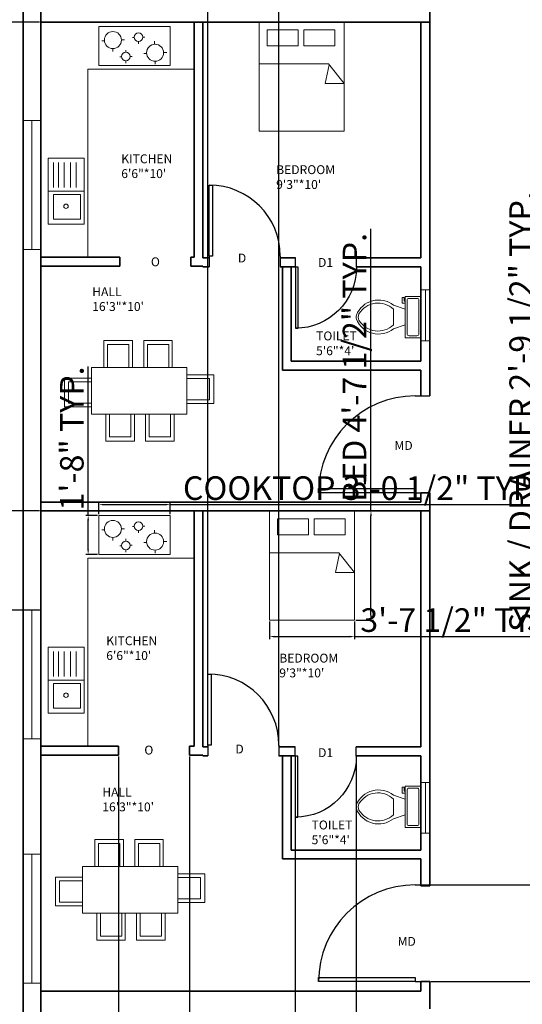
# Model space of a CAD drawing. Units: inches. Extents: x 1947 to 2903, y 1974 to 3472.
# Tile 3 of 5: x 2267 to 2523, y 2335 to 2836. Entities that reach past the tile are written whole.
import ezdxf

# ---------------------------------------------------------------- set-up
doc = ezdxf.new("R2010")
doc.units = ezdxf.units.IN
for name, color, linetype, lineweight in [('A-ANNO-DIMS', 2, 'Continuous', 18), ('A-ANNO-TEXT', 7, 'Continuous', 18), ('A-AREA-IDEN', 7, 'Continuous', 18), ('A-DOOR', 3, 'Continuous', 25), ('A-EQPM', 8, 'Continuous', 18), ('A-FLOR-CASE', 8, 'Continuous', 18), ('A-FLOR-FIXT', 9, 'Continuous', 18), ('A-FURN', 8, 'Continuous', 18), ('A-GLAZ', 4, 'Continuous', 18), ('A-GLAZ-VENT', 4, 'Continuous', 18), ('A-WALL', 7, 'Continuous', 35)]:
    doc.layers.add(name, color=color, linetype=linetype, lineweight=lineweight)
doc.styles.get("Standard").update_dxf_attribs({"font": 'arial.ttf'})
doc.dimstyles.new('ISO-25', dxfattribs={"dimtxt": 12, "dimasz": 2.5, "dimexe": 1.25, "dimexo": 0.625, "dimtad": 1, "dimdec": 0, "dimlunit": 4, "dimtxsty": 'Standard', "dimcen": 2.5, "dimadec": 0, "dimazin": 0, "dimtfac": 1, "dimtdec": 0, "dimtmove": 0, "dimatfit": 3, "dimfxl": 1, "dimarcsym": 0})

# ---------------------------------------------------------------- blocks, each defined once
blk = doc.blocks.new('*U2')
for p, q in [((0, 0), (0, -6)), ((40, 0), (40, -6))]:
    blk.add_line(p, q)
blk.add_lwpolyline([(0, 0), (0, 40), (1.75, 40), (1.75, 0)], close=True)
blk.add_arc((0, 0), 40, 0, 90)
blk = doc.blocks.new('*U4')
for p, q in [((9.5, -6), (9.5, -2)), ((-10, -8.5), (-8, -8.5)), ((-10, -9.5), (-10, -8.5)), ((-7, -9.5), (-10, -9.5)), ((-8, -8.5), (-8, -8)), ((-7, -8), (-7, -9.5)), ((-4, -8), (-6, -14)), ((4, -8), (6, -14)), ((4, -14), (-4, -14))]:
    blk.add_line(p, q)
blk.add_lwpolyline([(10.5, -8), (10.5, 0), (-10.5, 0), (-10.5, -8)], close=True)
for points in [[(-9.5, -2), (-9.5, -6)], [(8.5, -1), (-8.5, -1)], [(-8.5, -7), (8.5, -7)]]:
    blk.add_lwpolyline(points)
for centre, radius, start, end in [((-8.62, -1.88), 0.884, 81.8699, 188.1301), ((8.62, -1.88), 0.884, 351.8699, 98.1301), ((-8.62, -6.12), 0.884, 171.8699, 278.1301), ((8.62, -6.12), 0.884, 261.8699, 8.1301), ((3.52, -21.58), 12.17, 141.4691, 247.9714), ((4.2, -21.82), 11.33, 136.3677, 238.9468), ((-3.52, -21.58), 12.17, 292.0284, 38.5307), ((-4.2, -21.82), 11.33, 301.053, 43.6321), ((0, -27.88), 4, 245.7318, 294.2682), ((0, -29), 4, 254.8605, 285.1395)]:
    blk.add_arc(centre, radius, start, end)
blk = doc.blocks.new('*D6')
at = {"layer": 'A-ANNO-DIMS', "color": 0, "lineweight": -2, "transparency": 16777216}
for p, q in [((2268.49, 3341.41), (2191.31, 3341.41)), ((2192.56, 3338.91), (2192.56, 2230.91)), ((2268.49, 2228.41), (2191.31, 2228.41))]:
    blk.add_line(p, q, dxfattribs=at)
at = {"layer": 'A-ANNO-DIMS', "color": 0, "lineweight": 100, "transparency": 16777216}
for points in [[(2192.15, 3338.91), (2192.98, 3338.91), (2192.56, 3341.41)], [(2192.15, 2230.91), (2192.98, 2230.91), (2192.56, 2228.41)]]:
    blk.add_solid(points, dxfattribs=at)
at = {"layer": 'Defpoints', "color": 0, "lineweight": 100, "transparency": 16777216}
for p in [(2269.11, 3341.41), (2192.56, 2228.41), (2269.11, 2228.41)]:
    blk.add_point(p, dxfattribs=at)
at = {"layer": 'A-ANNO-DIMS', "color": 0, "transparency": 16777216, "insert": (2185.81, 2784.91), "char_height": 12, "attachment_point": 5, "rotation": 90}
blk.add_mtext('92\'-9"', dxfattribs=at)
blk = doc.blocks.new('BED-TWO-PILLOWS')
for p, q in [((0, 34.29), (35.37, 34.29)), ((33.59, 24.29), (35.7, 33.87)), ((35.37, 34.29), (43.32, 24.29)), ((43.32, 24.29), (33.59, 24.29))]:
    blk.add_line(p, q)
for points in [[(0, 55.57), (43.32, 55.57), (43.32, 0), (0, 0)], [(4.07, 51.54), (19.88, 51.54), (19.88, 43.48), (4.07, 43.48)], [(22.78, 51.54), (38.59, 51.54), (38.59, 43.48), (22.78, 43.48)]]:
    blk.add_lwpolyline(points, close=True)
blk = doc.blocks.new('DINING-SET-6')
for p, q in [((20.16, 37.5), (20.16, 51.24)), ((20.16, 51.24), (34.7, 51.24)), ((34.7, 51.24), (34.7, 37.5)), ((40.4, 37.5), (40.4, 51.24)), ((40.4, 51.24), (54.94, 51.24)), ((54.94, 51.24), (54.94, 37.5)), ((13.74, 31.99), (0, 31.99)), ((0, 31.99), (0, 17.45)), ((62.33, 33.71), (76.07, 33.71)), ((76.07, 33.71), (76.07, 19.17)), ((0, 17.45), (13.74, 17.45)), ((76.07, 19.17), (62.33, 19.17)), ((21.08, 13.74), (21.08, 0)), ((35.62, 0), (35.62, 13.74)), ((41.32, 13.74), (41.32, 0)), ((55.86, 0), (55.86, 13.74)), ((21.08, 0), (35.62, 0)), ((41.32, 0), (55.86, 0))]:
    blk.add_line(p, q)
for points in [[(22.02, 37.5), (32.87, 37.5), (32.87, 49.12), (22.02, 49.12)], [(42.26, 37.5), (53.11, 37.5), (53.11, 49.12), (42.26, 49.12)], [(13.74, 13.74), (62.33, 13.74), (62.33, 37.5), (13.74, 37.5)], [(13.74, 30.13), (13.74, 19.28), (2.12, 19.28), (2.12, 30.13)], [(62.33, 31.85), (62.33, 21), (73.95, 21), (73.95, 31.85)], [(22.94, 13.74), (33.79, 13.74), (33.79, 2.12), (22.94, 2.12)], [(43.18, 13.74), (54.03, 13.74), (54.03, 2.12), (43.18, 2.12)]]:
    blk.add_lwpolyline(points, close=True)
blk = doc.blocks.new('SINK-DRAINER-5')
for p, q in [((2.58, 18.66), (2.58, 31.31)), ((5.19, 18.66), (5.19, 31.31)), ((8.1, 18.66), (8.1, 31.31)), ((11.22, 18.66), (11.22, 31.31)), ((14.13, 18.66), (14.13, 31.31)), ((0, 16.81), (18.23, 16.81))]:
    blk.add_line(p, q)
for points in [[(0, 0), (18.23, 0), (18.23, 33.61), (0, 33.61)], [(2.68, 15.14), (16.44, 15.14), (16.44, 2.49), (2.68, 2.49)]]:
    blk.add_lwpolyline(points, close=True)
blk.add_circle((9.01, 9.12), 1.11)
blk = doc.blocks.new('WINDOW-EXTERIOR')
blk.add_line((0, 4.5), (65.51, 4.5))
blk.add_lwpolyline([(0, 0), (65.51, 0), (65.51, 9), (0, 9)], close=True)
blk = doc.blocks.new('VENT-TOILET')
blk.add_line((2.25, 0), (2.25, 25.89))
blk.add_lwpolyline([(0, 25.89), (4.5, 25.89), (4.5, 0), (0, 0)], close=True)
blk = doc.blocks.new('COOKTOP-4-BURNER-B')
for p, q in [((2.85, 12.63), (1.48, 12.63)), ((11.47, 13.09), (13.05, 13.09)), ((17.95, 14.27), (17.07, 14.27)), ((20.18, 12.22), (20.18, 11.07)), ((22.35, 14.5), (23.33, 14.5)), ((28.35, 10.88), (28.35, 12.39)), ((7.15, 8.69), (7.15, 7.15)), ((13.68, 6.8), (13.68, 7.94)), ((24.3, 6.18), (22.93, 6.18)), ((32.92, 6.64), (34.51, 6.64)), ((11.52, 4.44), (10.65, 4.44)), ((13.75, 2.4), (13.75, 1.25)), ((15.92, 4.68), (16.91, 4.68)), ((28.6, 2.24), (28.6, 0.71))]:
    blk.add_line(p, q)
blk.add_lwpolyline([(0, 0), (36.35, 0), (36.35, 19.93), (0, 19.93)], close=True)
for centre, radius in [((7.15, 13.01), 4.32), ((20.14, 14.42), 2.2), ((28.6, 6.56), 4.32), ((13.72, 4.6), 2.2)]:
    blk.add_circle(centre, radius)
blk = doc.blocks.new('*D19')
at = {"layer": 'A-ANNO-DIMS', "color": 0, "lineweight": -2, "transparency": 16777216}
for p, q in [((2446.19, 2586.39), (2446.19, 2729.84)), ((2438.48, 2586.39), (2447.44, 2586.39)), ((2446.19, 2533.33), (2446.19, 2583.89)), ((2438.48, 2530.83), (2447.44, 2530.83))]:
    blk.add_line(p, q, dxfattribs=at)
at = {"layer": 'A-ANNO-DIMS', "color": 0, "lineweight": 100, "transparency": 16777216}
for points in [[(2445.77, 2583.89), (2446.61, 2583.89), (2446.19, 2586.39)], [(2445.77, 2533.33), (2446.61, 2533.33), (2446.19, 2530.83)]]:
    blk.add_solid(points, dxfattribs=at)
at = {"layer": 'Defpoints', "color": 0, "lineweight": 100, "transparency": 16777216}
for p in [(2437.85, 2586.39), (2446.19, 2586.39), (2437.85, 2530.83)]:
    blk.add_point(p, dxfattribs=at)
at = {"layer": 'A-ANNO-DIMS', "color": 0, "transparency": 16777216, "insert": (2439.36, 2659.37), "char_height": 12, "attachment_point": 5, "rotation": 90}
blk.add_mtext('BED 4\'-7 1/2" TYP.', dxfattribs=at)
blk = doc.blocks.new('*D20')
at = {"layer": 'A-ANNO-DIMS', "color": 0, "lineweight": -2, "transparency": 16777216}
for p, q in [((2394.54, 2530.2), (2394.54, 2521.24)), ((2437.85, 2530.2), (2437.85, 2521.24)), ((2397.04, 2522.49), (2435.35, 2522.49)), ((2437.85, 2522.49), (2542.7, 2522.49))]:
    blk.add_line(p, q, dxfattribs=at)
at = {"layer": 'A-ANNO-DIMS', "color": 0, "lineweight": 100, "transparency": 16777216}
for points in [[(2397.04, 2522.91), (2397.04, 2522.07), (2394.54, 2522.49)], [(2435.35, 2522.91), (2435.35, 2522.07), (2437.85, 2522.49)]]:
    blk.add_solid(points, dxfattribs=at)
at = {"layer": 'Defpoints', "color": 0, "lineweight": 100, "transparency": 16777216}
for p in [(2394.54, 2530.83), (2437.85, 2530.83), (2437.85, 2522.49)]:
    blk.add_point(p, dxfattribs=at)
at = {"layer": 'A-ANNO-DIMS', "color": 0, "transparency": 16777216, "insert": (2491.53, 2529.32), "char_height": 12, "attachment_point": 5}
blk.add_mtext('3\'-7 1/2" TYP.', dxfattribs=at)
blk = doc.blocks.new('*D29')
at = {"layer": 'A-ANNO-DIMS', "color": 0, "lineweight": -2, "transparency": 16777216}
for p, q in [((2531.02, 2516.69), (2531.02, 2754.7)), ((2535.44, 2516.69), (2529.77, 2516.69)), ((2531.02, 2485.58), (2531.02, 2514.19)), ((2535.44, 2483.08), (2529.77, 2483.08))]:
    blk.add_line(p, q, dxfattribs=at)
at = {"layer": 'A-ANNO-DIMS', "color": 0, "lineweight": 100, "transparency": 16777216}
for points in [[(2530.61, 2514.19), (2531.44, 2514.19), (2531.02, 2516.69)], [(2530.61, 2485.58), (2531.44, 2485.58), (2531.02, 2483.08)]]:
    blk.add_solid(points, dxfattribs=at)
at = {"layer": 'Defpoints', "color": 0, "lineweight": 100, "transparency": 16777216}
for p in [(2531.02, 2516.69), (2536.07, 2516.69), (2536.07, 2483.08)]:
    blk.add_point(p, dxfattribs=at)
at = {"layer": 'A-ANNO-DIMS', "color": 0, "transparency": 16777216, "insert": (2524.19, 2636.95), "char_height": 12, "attachment_point": 5, "rotation": 90}
blk.add_mtext('SINK / DRAINER 2\'-9 1/2" TYP.', dxfattribs=at)
blk = doc.blocks.new('*D31')
at = {"layer": 'A-ANNO-DIMS', "color": 0, "lineweight": -2, "transparency": 16777216}
for p, q in [((2307.69, 2584.79), (2307.69, 2590.86)), ((2310.19, 2589.61), (2341.53, 2589.61)), ((2344.03, 2584.79), (2344.03, 2590.86)), ((2344.03, 2589.61), (2537.24, 2589.61))]:
    blk.add_line(p, q, dxfattribs=at)
at = {"layer": 'A-ANNO-DIMS', "color": 0, "lineweight": 100, "transparency": 16777216}
for points in [[(2310.19, 2590.03), (2310.19, 2589.2), (2307.69, 2589.61)], [(2341.53, 2590.03), (2341.53, 2589.2), (2344.03, 2589.61)]]:
    blk.add_solid(points, dxfattribs=at)
at = {"layer": 'Defpoints', "color": 0, "lineweight": 100, "transparency": 16777216}
for p in [(2344.03, 2589.61), (2307.69, 2584.16), (2344.03, 2584.16)]:
    blk.add_point(p, dxfattribs=at)
at = {"layer": 'A-ANNO-DIMS', "color": 0, "transparency": 16777216, "insert": (2441.89, 2596.45), "char_height": 12, "attachment_point": 5}
blk.add_mtext('COOKTOP 3\'-0 1/2" TYP.', dxfattribs=at)
blk = doc.blocks.new('*D32')
at = {"layer": 'A-ANNO-DIMS', "color": 0, "lineweight": -2, "transparency": 16777216}
for p, q in [((2302.23, 2584.16), (2302.23, 2659.93)), ((2307.06, 2584.16), (2300.98, 2584.16)), ((2302.23, 2566.73), (2302.23, 2581.66)), ((2307.06, 2564.23), (2300.98, 2564.23))]:
    blk.add_line(p, q, dxfattribs=at)
at = {"layer": 'A-ANNO-DIMS', "color": 0, "lineweight": 100, "transparency": 16777216}
for points in [[(2301.82, 2581.66), (2302.65, 2581.66), (2302.23, 2584.16)], [(2301.82, 2566.73), (2302.65, 2566.73), (2302.23, 2564.23)]]:
    blk.add_solid(points, dxfattribs=at)
at = {"layer": 'Defpoints', "color": 0, "lineweight": 100, "transparency": 16777216}
for p in [(2302.23, 2584.16), (2307.69, 2584.16), (2307.69, 2564.23)]:
    blk.add_point(p, dxfattribs=at)
at = {"layer": 'A-ANNO-DIMS', "color": 0, "transparency": 16777216, "insert": (2295.48, 2623.3), "char_height": 12, "attachment_point": 5, "rotation": 90}
blk.add_mtext('1\'-8" TYP.', dxfattribs=at)
blk = doc.blocks.new('*D38')
at = {"layer": 'A-ANNO-DIMS', "color": 0, "lineweight": -2, "transparency": 16777216}
for p, q in [((2277.49, 2835.06), (1970.32, 2835.06)), ((1971.57, 2588.89), (1971.57, 2832.56)), ((2277.49, 2586.39), (1970.32, 2586.39))]:
    blk.add_line(p, q, dxfattribs=at)
at = {"layer": 'A-ANNO-DIMS', "color": 0, "lineweight": 100, "transparency": 16777216}
for points in [[(1971.16, 2832.56), (1971.99, 2832.56), (1971.57, 2835.06)], [(1971.16, 2588.89), (1971.99, 2588.89), (1971.57, 2586.39)]]:
    blk.add_solid(points, dxfattribs=at)
at = {"layer": 'Defpoints', "color": 0, "lineweight": 100, "transparency": 16777216}
for p in [(1971.57, 2835.06), (2278.11, 2835.06), (2278.11, 2586.39)]:
    blk.add_point(p, dxfattribs=at)
at = {"layer": 'A-ANNO-DIMS', "color": 0, "transparency": 16777216, "insert": (1964.74, 2710.73), "char_height": 12, "attachment_point": 5, "rotation": 90}
blk.add_mtext('20\'-8 1/2"', dxfattribs=at)
blk = doc.blocks.new('*D39')
at = {"layer": 'A-ANNO-DIMS', "color": 0, "lineweight": -2, "transparency": 16777216}
for p, q in [((2476.73, 2396.2), (2903.22, 2396.2)), ((2901.97, 2349.5), (2901.97, 2393.7)), ((2476.73, 2347), (2903.22, 2347))]:
    blk.add_line(p, q, dxfattribs=at)
at = {"layer": 'A-ANNO-DIMS', "color": 0, "lineweight": 100, "transparency": 16777216}
for points in [[(2901.55, 2393.7), (2902.39, 2393.7), (2901.97, 2396.2)], [(2901.55, 2349.5), (2902.39, 2349.5), (2901.97, 2347)]]:
    blk.add_solid(points, dxfattribs=at)
at = {"layer": 'Defpoints', "color": 0, "lineweight": 100, "transparency": 16777216}
for p in [(2476.11, 2396.2), (2901.97, 2396.2), (2476.11, 2347)]:
    blk.add_point(p, dxfattribs=at)
at = {"layer": 'A-ANNO-DIMS', "color": 0, "transparency": 16777216, "insert": (2895.32, 2371.6), "char_height": 12, "attachment_point": 5, "rotation": 90}
blk.add_mtext('4\'-1"', dxfattribs=at)
blk = doc.blocks.new('*D40')
at = {"layer": 'A-ANNO-DIMS', "color": 0, "lineweight": -2, "transparency": 16777216}
for p, q in [((2363.18, 2467.02), (2363.18, 3458.67)), ((2365.68, 3457.42), (2396.82, 3457.42)), ((2399.32, 2467.02), (2399.32, 3458.67))]:
    blk.add_line(p, q, dxfattribs=at)
at = {"layer": 'A-ANNO-DIMS', "color": 0, "lineweight": 100, "transparency": 16777216}
for points in [[(2365.68, 3457.83), (2365.68, 3457), (2363.18, 3457.42)], [(2396.82, 3457.83), (2396.82, 3457), (2399.32, 3457.42)]]:
    blk.add_solid(points, dxfattribs=at)
at = {"layer": 'Defpoints', "color": 0, "lineweight": 100, "transparency": 16777216}
for p in [(2399.32, 3457.42), (2363.18, 2466.39), (2399.32, 2466.39)]:
    blk.add_point(p, dxfattribs=at)
at = {"layer": 'A-ANNO-DIMS', "color": 0, "transparency": 16777216, "insert": (2381.25, 3464.17), "char_height": 12, "attachment_point": 5}
blk.add_mtext('3\'-0"', dxfattribs=at)
blk = doc.blocks.new('*D41')
at = {"layer": 'A-ANNO-DIMS', "color": 0, "lineweight": -2, "transparency": 16777216}
for p, q in [((2407.63, 2461.27), (2407.63, 1983.7)), ((2438.73, 2461.27), (2438.73, 1983.7)), ((2410.13, 1984.95), (2436.23, 1984.95)), ((2438.73, 1984.95), (2474.58, 1984.95))]:
    blk.add_line(p, q, dxfattribs=at)
at = {"layer": 'A-ANNO-DIMS', "color": 0, "lineweight": 100, "transparency": 16777216}
for points in [[(2410.13, 1985.36), (2410.13, 1984.53), (2407.63, 1984.95)], [(2436.23, 1985.36), (2436.23, 1984.53), (2438.73, 1984.95)]]:
    blk.add_solid(points, dxfattribs=at)
at = {"layer": 'Defpoints', "color": 0, "lineweight": 100, "transparency": 16777216}
for p in [(2407.63, 2461.89), (2438.73, 2461.89), (2438.73, 1984.95)]:
    blk.add_point(p, dxfattribs=at)
at = {"layer": 'A-ANNO-DIMS', "color": 0, "transparency": 16777216, "insert": (2457.91, 1991.6), "char_height": 12, "attachment_point": 5}
blk.add_mtext('2\'-7"', dxfattribs=at)
blk = doc.blocks.new('*D42')
at = {"layer": 'A-ANNO-DIMS', "color": 0, "lineweight": -2, "transparency": 16777216}
for p, q in [((2317.62, 2461.59), (2317.62, 1983.7)), ((2353.75, 2461.59), (2353.75, 1983.7)), ((2320.12, 1984.95), (2351.25, 1984.95))]:
    blk.add_line(p, q, dxfattribs=at)
at = {"layer": 'A-ANNO-DIMS', "color": 0, "lineweight": 100, "transparency": 16777216}
for points in [[(2320.12, 1985.36), (2320.12, 1984.53), (2317.62, 1984.95)], [(2351.25, 1985.36), (2351.25, 1984.53), (2353.75, 1984.95)]]:
    blk.add_solid(points, dxfattribs=at)
at = {"layer": 'Defpoints', "color": 0, "lineweight": 100, "transparency": 16777216}
for p in [(2317.62, 2462.22), (2353.75, 2462.22), (2353.75, 1984.95)]:
    blk.add_point(p, dxfattribs=at)
at = {"layer": 'A-ANNO-DIMS', "color": 0, "transparency": 16777216, "insert": (2335.68, 1991.7), "char_height": 12, "attachment_point": 5}
blk.add_mtext('3\'-0"', dxfattribs=at)
blk = doc.blocks.new('*D45')
at = {"layer": 'A-ANNO-DIMS', "color": 0, "lineweight": -2, "transparency": 16777216}
for p, q in [((2277.49, 2586.39), (1970.32, 2586.39)), ((1971.57, 2583.89), (1971.57, 2538.49)), ((2277.49, 2535.99), (1970.32, 2535.99)), ((1971.57, 2535.99), (1971.57, 2471.89))]:
    blk.add_line(p, q, dxfattribs=at)
at = {"layer": 'A-ANNO-DIMS', "color": 0, "lineweight": 100, "transparency": 16777216}
for points in [[(1971.16, 2583.89), (1971.99, 2583.89), (1971.57, 2586.39)], [(1971.16, 2538.49), (1971.99, 2538.49), (1971.57, 2535.99)]]:
    blk.add_solid(points, dxfattribs=at)
at = {"layer": 'Defpoints', "color": 0, "lineweight": 100, "transparency": 16777216}
for p in [(2278.11, 2586.39), (1971.57, 2535.99), (2278.11, 2535.99)]:
    blk.add_point(p, dxfattribs=at)
at = {"layer": 'A-ANNO-DIMS', "color": 0, "transparency": 16777216, "insert": (1964.74, 2502.69), "char_height": 12, "attachment_point": 5, "rotation": 90}
blk.add_mtext('4\'-2 1/2"', dxfattribs=at)
blk = doc.blocks.new('*D46')
at = {"layer": 'A-ANNO-DIMS', "color": 0, "lineweight": -2, "transparency": 16777216}
for p, q in [((2278.11, 2461.59), (2278.11, 1983.7)), ((2317.62, 2461.59), (2317.62, 1983.7)), ((2280.61, 1984.95), (2315.12, 1984.95)), ((2317.62, 1984.95), (2381.22, 1984.95))]:
    blk.add_line(p, q, dxfattribs=at)
at = {"layer": 'A-ANNO-DIMS', "color": 0, "lineweight": 100, "transparency": 16777216}
for points in [[(2280.61, 1985.36), (2280.61, 1984.53), (2278.11, 1984.95)], [(2315.12, 1985.36), (2315.12, 1984.53), (2317.62, 1984.95)]]:
    blk.add_solid(points, dxfattribs=at)
at = {"layer": 'Defpoints', "color": 0, "lineweight": 100, "transparency": 16777216}
for p in [(2278.11, 2462.22), (2317.62, 2462.22), (2317.62, 1984.95)]:
    blk.add_point(p, dxfattribs=at)
at = {"layer": 'A-ANNO-DIMS', "color": 0, "transparency": 16777216, "insert": (2350.67, 1991.78), "char_height": 12, "attachment_point": 5}
blk.add_mtext('3\'-3 1/2"', dxfattribs=at)

msp = doc.modelspace()

# ---------------------------------------------------------------- linework, layer by layer
at = {"layer": 'A-FLOR-CASE'}
for p, q in [((2302.11, 2715.39), (2302.11, 2811.06)), ((2356.11, 2811.06), (2302.11, 2811.06)), ((2278.11, 2715.39), (2302.11, 2715.39)), ((2302.11, 2466.72), (2302.11, 2562.39)), ((2356.11, 2562.39), (2302.11, 2562.39)), ((2278.11, 2466.72), (2302.11, 2466.72))]:
    msp.add_line(p, q, dxfattribs=at)
at = {"layer": 'A-WALL'}
for p, q in [((2476.11, 2848.84), (2476.11, 2835.06)), ((2278.11, 2835.06), (2476.11, 2835.06)), ((2278.11, 2835.06), (2476.11, 2835.06)), ((2356.11, 2835.06), (2356.11, 2715.39)), ((2360.61, 2835.06), (2360.61, 2715.06)), ((2360.61, 2835.06), (2471.61, 2835.06)), ((2471.61, 2835.06), (2471.61, 2715.06)), ((2476.11, 2835.06), (2476.11, 2710.56)), ((2318.32, 2715.39), (2278.11, 2715.39)), ((2316.73, 2715.39), (2278.11, 2715.39)), ((2318.32, 2710.89), (2318.32, 2715.39)), ((2356.11, 2715.39), (2354.46, 2715.39)), ((2354.46, 2710.89), (2354.46, 2715.39)), ((2363.89, 2715.06), (2360.61, 2715.06)), ((2407.74, 2715.06), (2400.02, 2715.06)), ((2471.61, 2715.06), (2438.84, 2715.06)), ((2278.11, 2710.89), (2278.11, 2590.89)), ((2318.32, 2710.89), (2278.11, 2710.89)), ((2360.61, 2710.89), (2354.46, 2710.89)), ((2363.89, 2710.56), (2360.61, 2710.56)), ((2407.74, 2710.56), (2400.02, 2710.56)), ((2401.11, 2658.06), (2401.11, 2710.56)), ((2405.61, 2662.56), (2405.61, 2710.56)), ((2471.61, 2710.56), (2438.84, 2710.56)), ((2471.61, 2710.56), (2471.61, 2662.56)), ((2476.11, 2710.56), (2476.11, 2644.87)), ((2471.61, 2662.56), (2405.61, 2662.56)), ((2471.61, 2658.06), (2401.11, 2658.06)), ((2471.61, 2658.06), (2471.61, 2644.87)), ((2471.61, 2658.06), (2471.61, 2644.87)), ((2471.61, 2595.67), (2471.61, 2590.89)), ((2471.61, 2595.67), (2476.11, 2595.67)), ((2471.61, 2595.67), (2471.61, 2590.89)), ((2476.11, 2595.67), (2476.11, 2586.39)), ((2476.11, 2595.67), (2476.11, 2586.39)), ((2278.11, 2590.89), (2471.61, 2590.89)), ((2278.11, 2590.89), (2471.61, 2590.89)), ((2278.11, 2586.39), (2476.11, 2586.39)), ((2278.11, 2586.39), (2476.11, 2586.39)), ((2356.11, 2586.39), (2356.11, 2466.72)), ((2360.61, 2586.39), (2360.61, 2466.39)), ((2360.61, 2586.39), (2471.61, 2586.39)), ((2471.61, 2586.39), (2471.61, 2466.39)), ((2476.11, 2586.39), (2476.11, 2461.89)), ((2317.62, 2466.72), (2278.11, 2466.72)), ((2316.73, 2466.72), (2278.11, 2466.72)), ((2317.62, 2462.22), (2317.62, 2466.72)), ((2356.11, 2466.72), (2353.75, 2466.72)), ((2353.75, 2462.22), (2353.75, 2466.72)), ((2363.18, 2466.39), (2360.61, 2466.39)), ((2407.63, 2466.39), (2399.32, 2466.39)), ((2471.61, 2466.39), (2438.73, 2466.39)), ((2278.11, 2462.22), (2278.11, 2342.22)), ((2317.62, 2462.22), (2278.11, 2462.22)), ((2360.61, 2462.22), (2353.75, 2462.22)), ((2363.18, 2461.89), (2360.61, 2461.89)), ((2407.63, 2461.89), (2399.32, 2461.89)), ((2401.11, 2409.39), (2401.11, 2461.89)), ((2405.61, 2413.89), (2405.61, 2461.89)), ((2471.61, 2461.89), (2438.73, 2461.89)), ((2471.61, 2461.89), (2471.61, 2413.89)), ((2476.11, 2461.89), (2476.11, 2395.75)), ((2471.61, 2413.89), (2405.61, 2413.89)), ((2471.61, 2409.39), (2401.11, 2409.39)), ((2471.61, 2409.39), (2471.61, 2395.75)), ((2471.61, 2409.39), (2471.61, 2395.75)), ((2471.61, 2395.75), (2476.11, 2395.75)), ((2471.61, 2347), (2471.61, 2342.22)), ((2471.61, 2347), (2476.11, 2347)), ((2471.61, 2347), (2471.61, 2342.22)), ((2476.11, 2347), (2476.11, 2337.72)), ((2476.11, 2347), (2476.11, 2333.22)), ((2278.11, 2342.22), (2471.61, 2342.22))]:
    msp.add_line(p, q, dxfattribs=at)
for points in [[(2269.11, 2228.41), (2737.11, 2228.41), (2737.11, 3341.41), (2269.11, 3341.41)], [(2278.11, 2237.41), (2728.11, 2237.41), (2728.11, 3332.41), (2278.11, 3332.41)]]:
    msp.add_lwpolyline(points, close=True, dxfattribs=at)

# ---------------------------------------------------------------- block references
at = {"layer": 'A-DOOR', "xscale": 0.9034599273514711, "yscale": 0.9034599273514711, "zscale": 0.9034599273514711}
for p in [(2363.89, 2715.98), (2363.18, 2467.31)]:
    msp.add_blockref('*U2', p, dxfattribs=at)
at = {"layer": 'A-DOOR'}
for p, xscale, yscale, zscale, rotation in [((2407.74, 2710.4), -0.7774936004188162, 0.7774936004188162, 0.7774936004188162, 180), ((2468.73, 2595.67), 1.23010588698369, 1.23010588698369, 1.23010588698369, 90.00000000000003), ((2407.63, 2461.73), -0.7774936004188162, 0.7774936004188162, 0.7774936004188162, 180), ((2468.73, 2347), 1.23010588698369, 1.23010588698369, 1.23010588698369, 90.00000000000003)]:
    msp.add_blockref('*U2', p, dxfattribs=dict(at, xscale=xscale, yscale=yscale, zscale=zscale, rotation=rotation))
at = {"layer": 'A-EQPM'}
for p in [(2307.69, 2812.9), (2307.69, 2564.23)]:
    msp.add_blockref('COOKTOP-4-BURNER-B', p, dxfattribs=at)
at = {"layer": 'A-FLOR-FIXT'}
for p in [(2281.94, 2732.23), (2281.94, 2483.56)]:
    msp.add_blockref('SINK-DRAINER-5', p, dxfattribs=at)
at = {"layer": 'A-FLOR-FIXT', "rotation": 270}
for p in [(2471.61, 2685.01), (2471.61, 2435.87)]:
    msp.add_blockref('*U4', p, dxfattribs=at)
at = {"layer": 'A-FURN'}
for name, p in [('BED-TWO-PILLOWS', (2389.22, 2779.5)), ('DINING-SET-6', (2290.12, 2621.93)), ('BED-TWO-PILLOWS', (2394.54, 2530.83)), ('DINING-SET-6', (2285.53, 2368.07))]:
    msp.add_blockref(name, p, dxfattribs=at)
at = {"layer": 'A-GLAZ'}
for p, rotation in [((2269.11, 2784.91), 269.9999999999994), ((2269.11, 2535.99), 269.9999999999995), ((2269.11, 2411.75), 269.9999999999993)]:
    msp.add_blockref('WINDOW-EXTERIOR', p, dxfattribs=dict(at, rotation=rotation))
at = {"layer": 'A-GLAZ-VENT'}
for p in [(2471.61, 2672.92), (2471.61, 2422.43)]:
    msp.add_blockref('VENT-TOILET', p, dxfattribs=at)

# ---------------------------------------------------------------- texts
at = {"layer": 'A-ANNO-TEXT', "attachment_point": 1}
for s, insert, char_height in [('O', (2334.17, 2715.37), 4.52), ('D', (2378.44, 2717.29), 4.52), ('D1', (2419.25, 2715.04), 4.519), ('MD', (2458.18, 2621.95), 4.519), ('O', (2330.83, 2467.05), 4.52), ('D', (2377.18, 2467.56), 4.52), ('D1', (2419.28, 2465.72), 4.519), ('MD', (2459.76, 2369.74), 4.519)]:
    msp.add_mtext_dynamic_manual_height_columns(s, width=35.9327, gutter_width=22.59, heights=[0], dxfattribs=dict(at, insert=insert, char_height=char_height))
at = {"layer": 'A-AREA-IDEN', "char_height": 4.519, "attachment_point": 1}
for s, insert in [('KITCHEN\\P6\'6"*10\'', (2319.08, 2767.77)), ('BEDROOM\\P9\'3"*10\'', (2397.94, 2762.23)), ('HALL\\P16\'3"*10\'', (2304.3, 2700.17)), ('TOILET\\P5\'6"*4\'', (2418.26, 2677.67)), ('KITCHEN\\P6\'6"*10\'', (2311.44, 2522.64)), ('BEDROOM\\P9\'3"*10\'', (2399.52, 2513.8)), ('HALL\\P16\'3"*10\'', (2309.43, 2445.66)), ('TOILET\\P5\'6"*4\'', (2415.97, 2428.95))]:
    msp.add_mtext_dynamic_manual_height_columns(s, width=35.9327, gutter_width=22.59, heights=[0], dxfattribs=dict(at, insert=insert))

# ---------------------------------------------------------------- dimensions: what is measured, and where the dimension line sits
at = {"layer": 'A-ANNO-DIMS'}
for base, p1, p2, picture, middle in [((2399.32, 3457.42), (2363.18, 2466.39), (2399.32, 2466.39), '*D40', (2381.25, 3464.17)), ((2317.62, 1984.95), (2278.11, 2462.22), (2317.62, 2462.22), '*D46', (2350.67, 1991.78)), ((2353.75, 1984.95), (2317.62, 2462.22), (2353.75, 2462.22), '*D42', (2335.68, 1991.7)), ((2438.73, 1984.95), (2407.63, 2461.89), (2438.73, 2461.89), '*D41', (2457.91, 1991.6))]:
    dim = msp.add_linear_dim(base=base, p1=p1, p2=p2, dimstyle='ISO-25', override={"dimdec": 1, "dimlfac": 1, "dimrnd": 0, "dimzin": 1, "dimdsep": 46, "dimlunit": 4, "dimfrac": 2}, dxfattribs=at)
    dim.commit()
    dim.dimension.update_dxf_attribs({"geometry": picture, "text_midpoint": middle})
for base, p1, p2, override, picture, middle in [((2192.56, 2228.41), (2269.11, 3341.41), (2269.11, 2228.41), {"dimclrd": 0, "dimclre": 0, "dimclrt": 0}, '*D6', (2185.81, 2784.91)), ((1971.57, 2835.06), (2278.11, 2586.39), (2278.11, 2835.06), {"dimdec": 1, "dimlfac": 1, "dimrnd": 0, "dimzin": 1, "dimdsep": 46, "dimlunit": 4, "dimfrac": 2}, '*D38', (1964.74, 2710.73)), ((1971.57, 2535.99), (2278.11, 2586.39), (2278.11, 2535.99), {"dimdec": 1, "dimlfac": 1, "dimrnd": 0, "dimzin": 1, "dimdsep": 46, "dimlunit": 4, "dimfrac": 2}, '*D45', (1964.74, 2502.69)), ((2901.97, 2396.2), (2476.11, 2347), (2476.11, 2396.2), {"dimdec": 1, "dimlfac": 1, "dimrnd": 0, "dimzin": 1, "dimdsep": 46, "dimlunit": 4, "dimfrac": 2}, '*D39', (2895.32, 2371.6))]:
    dim = msp.add_linear_dim(base=base, p1=p1, p2=p2, angle=90, dimstyle='ISO-25', override=override, dxfattribs=at)
    dim.commit()
    dim.dimension.update_dxf_attribs({"geometry": picture, "text_midpoint": middle})
for base, p1, p2, text, picture, middle in [((2531.02, 2516.69), (2536.07, 2483.08), (2536.07, 2516.69), 'SINK / DRAINER <> TYP.', '*D29', (2524.19, 2636.95)), ((2446.19, 2586.39), (2437.85, 2530.83), (2437.85, 2586.39), 'BED <> TYP.', '*D19', (2439.36, 2659.37)), ((2302.23, 2584.16), (2307.69, 2564.23), (2307.69, 2584.16), '<> TYP.', '*D32', (2295.48, 2623.3))]:
    dim = msp.add_linear_dim(base=base, p1=p1, p2=p2, angle=90, text=text, dimstyle='ISO-25', override={"dimdec": 1, "dimlfac": 1, "dimrnd": 0, "dimzin": 1, "dimdsep": 46, "dimlunit": 4, "dimfrac": 2}, dxfattribs=at)
    dim.commit()
    dim.dimension.update_dxf_attribs({"geometry": picture, "text_midpoint": middle})
for base, p1, p2, text, picture, middle in [((2344.03, 2589.61), (2307.69, 2584.16), (2344.03, 2584.16), 'COOKTOP <> TYP.', '*D31', (2441.89, 2596.45)), ((2437.85, 2522.49), (2394.54, 2530.83), (2437.85, 2530.83), '<> TYP.', '*D20', (2491.53, 2529.32))]:
    dim = msp.add_linear_dim(base=base, p1=p1, p2=p2, text=text, dimstyle='ISO-25', override={"dimdec": 1, "dimlfac": 1, "dimrnd": 0, "dimzin": 1, "dimdsep": 46, "dimlunit": 4, "dimfrac": 2}, dxfattribs=at)
    dim.commit()
    dim.dimension.update_dxf_attribs({"geometry": picture, "text_midpoint": middle})

doc.saveas('drawing.dxf')
